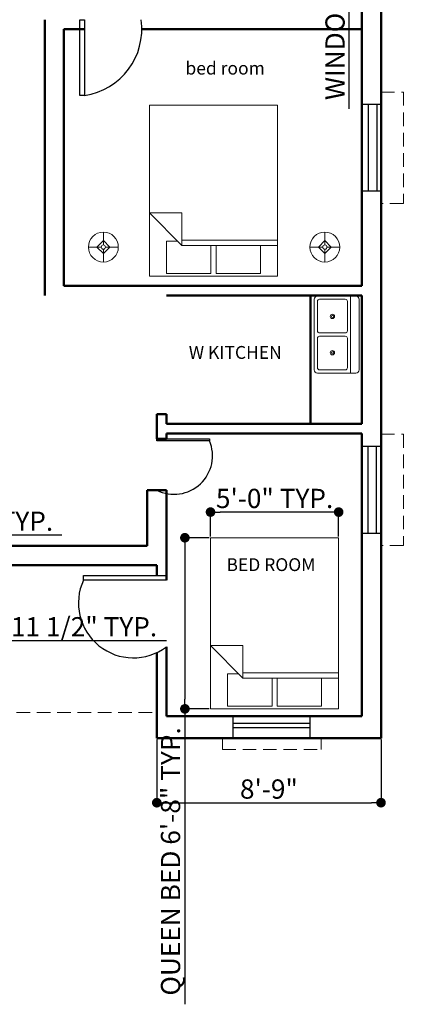
# Model space of a CAD drawing. Units: inches. Extents: x 2050 to 6806, y 2092 to 5743.
# Tile 5 of 8: x 3382 to 3567, y 2211 to 2671. Entities that reach past the tile are written whole.
import ezdxf

# ---------------------------------------------------------------- set-up
doc = ezdxf.new("R2010")
doc.units = ezdxf.units.IN
doc.linetypes.add('HIDDEN', pattern=[9.525, 6.35, -3.175])
for name, color, linetype, lineweight in [('A-ANNO-DIMS', 2, 'Continuous', 18), ('A-AREA-IDEN', 7, 'Continuous', 18), ('A-DOOR', 2, 'Continuous', 25), ('A-FLOR-FIXT', 4, 'Continuous', 18), ('A-FLOR-OVHD', 30, 'HIDDEN', 18), ('A-FURN', 5, 'Continuous', 18), ('A-GLAZ', 6, 'Continuous', 25), ('A-WALL', 7, 'Continuous', 50)]:
    doc.layers.add(name, color=color, linetype=linetype, lineweight=lineweight)
doc.styles.get("Standard").update_dxf_attribs({"font": 'arial.ttf'})
doc.dimstyles.new('ISO-25', dxfattribs={"dimtxt": 9, "dimasz": 4.5, "dimexe": 1.25, "dimexo": 0.625, "dimtad": 1, "dimdec": 1, "dimlunit": 4, "dimtxsty": 'Standard', "dimblk": 'DOT', "dimcen": 2.5, "dimadec": 0, "dimazin": 0, "dimtfac": 1, "dimtdec": 1, "dimtmove": 0, "dimatfit": 3, "dimldrblk": 'ARCHTICK', "dimfxl": 1, "dimarcsym": 0})

# ---------------------------------------------------------------- blocks, each defined once
blk = doc.blocks.new('Bed - Queen')
for p, q in [((0, -80.00003), (0, 0)), ((0, 0), (59.99999, 0)), ((59.99999, 0), (59.99999, -80.00003)), ((7.99999, -1.2), (28.79998, -1.2)), ((7.99999, -14.4), (7.99999, -1.2)), ((28.79998, -1.2), (28.79998, -14.4)), ((31.19999, -1.2), (51.99999, -1.2)), ((31.19999, -14.4), (31.19999, -1.2)), ((51.99999, -1.2), (51.99999, -16.4)), ((0, -14.4), (44.8, -14.4)), ((44.8, -16.8), (0, -16.8)), ((59.99999, -29.6), (44.8, -14.4)), ((44.8, -14.4), (44.8, -29.6)), ((51.99999, -16.4), (46.79936, -16.4)), ((44.8, -29.6), (59.99999, -29.6)), ((59.99999, -80.00003), (0, -80.00003))]:
    blk.add_line(p, q)
blk = doc.blocks.new('Lamp - Table')
for p, q in [((0, 7), (0, 1)), ((-1, 0), (-7, 0)), ((0, 3), (-3, 0)), ((-3, 0), (0, -3)), ((3, 0), (0, 3)), ((0, -3), (3, 0)), ((1, 0), (7, 0)), ((0, -1), (0, -7))]:
    blk.add_line(p, q)
for radius in [7, 1]:
    blk.add_circle((0, 0), radius)
blk = doc.blocks.new('Sink-double - 36 in top')
for p, q in [((-18, -4), (18, -4)), ((-0.75, -18.5), (-0.75, -6.5)), ((0.75, -6.5), (0.75, -18.5))]:
    blk.add_line(p, q)
for points in [[(-16.5, 0), (16.5, 0)], [(-18, -19.5), (-18, -1.5)], [(18, -1.5), (18, -19.5)], [(-16.5, -18.5), (-16.5, -6.5)], [(-15.5, -5.5), (-1.75, -5.5)], [(1.75, -5.5), (15.5, -5.5)], [(16.5, -6.5), (16.5, -18.5)], [(16.5, -21), (-16.5, -21)], [(-1.75, -19.5), (-15.5, -19.5)], [(15.5, -19.5), (1.75, -19.5)]]:
    blk.add_lwpolyline(points)
for centre, radius in [((-8.5, -12.5), 1), ((-8.5, -12.5), 0.5), ((8.5, -12.5), 1), ((8.5, -12.5), 0.5)]:
    blk.add_circle(centre, radius)
for centre, radius, start, end in [((-16.5, -1.5), 1.5, 90, 180), ((16.5, -1.5), 1.5, 0, 90), ((-15.5, -6.5), 1, 90, 180), ((-1.75, -6.5), 1, 0, 90), ((1.75, -6.5), 1, 90, 180), ((15.5, -6.5), 1, 0, 90), ((-16.5, -19.5), 1.5, 180, 270), ((-15.5, -18.5), 1, 180, 270), ((-1.75, -18.5), 1, 270, 0), ((1.75, -18.5), 1, 180, 270), ((15.5, -18.5), 1, 270, 0), ((16.5, -19.5), 1.5, 270, 0)]:
    blk.add_arc(centre, radius, start, end)
blk = doc.blocks.new('_Dot')
at = {"color": 0, "linetype": 'ByBlock', "lineweight": -2}
blk.add_line((-0.5, 0), (-1, 0), dxfattribs=at)
at = {"color": 0, "linetype": 'ByBlock', "const_width": 0.5}
blk.add_lwpolyline([(-0.25, 0, 1), (0.25, 0, 1)], format="xyb", close=True, dxfattribs=at)
blk = doc.blocks.new('*D43')
at = {"layer": 'A-ANNO-DIMS', "color": 0, "lineweight": -2, "transparency": 16777216}
for p, q in [((3446.67, 2334.81), (3446.67, 2303.96)), ((3551.67, 2334.81), (3551.67, 2303.96)), ((3451.17, 2305.21), (3547.17, 2305.21))]:
    blk.add_line(p, q, dxfattribs=at)
at = {"layer": 'Defpoints', "color": 0, "transparency": 16777216}
for p in [(3446.67, 2335.44), (3551.67, 2335.44), (3551.67, 2305.21)]:
    blk.add_point(p, dxfattribs=at)
at = {"layer": 'A-ANNO-DIMS', "color": 0, "lineweight": -2, "transparency": 16777216, "xscale": 4.5, "yscale": 4.5, "zscale": 4.5, "rotation": 180}
blk.add_blockref('_Dot', (3446.67, 2305.21), dxfattribs=at)
at = {"layer": 'A-ANNO-DIMS', "color": 0, "lineweight": -2, "transparency": 16777216, "xscale": 4.5, "yscale": 4.5, "zscale": 4.5}
blk.add_blockref('_Dot', (3551.67, 2305.21), dxfattribs=at)
at = {"layer": 'A-ANNO-DIMS', "color": 0, "transparency": 16777216, "insert": (3499.17, 2310.43), "char_height": 9, "attachment_point": 5}
blk.add_mtext('8\'-9"', dxfattribs=at)
blk = doc.blocks.new('_ArchTick')
at = {"color": 0, "linetype": 'ByBlock', "const_width": 0.15}
blk.add_lwpolyline([(-0.5, -0.5), (0.5, 0.5)], dxfattribs=at)
blk = doc.blocks.new('DOOR-750')
blk.add_lwpolyline([(28.97, 0), (26.83, 0), (26.83, 35.38), (28.97, 35.38)], close=True)
blk.add_arc((31.25, 4.42), 31.27, 98.1233, 188.1233)
blk = doc.blocks.new('WIN-1050')
for p, q in [((0, 40.58), (9, 40.58)), ((2.5, 0), (2.5, 40.58)), ((6.5, 0), (6.5, 40.58)), ((0, 0), (9, 0))]:
    blk.add_line(p, q)
blk = doc.blocks.new('SUNSHADE-A')
for p, q in [((0, 52.08), (10.45, 52.08)), ((10.45, 52.08), (10.45, 0)), ((10.45, 0), (0, 0))]:
    blk.add_line(p, q)
blk = doc.blocks.new('*D65')
at = {"layer": 'A-ANNO-DIMS', "color": 0, "lineweight": -2, "transparency": 16777216}
for p, q in [((3471.21, 2429.09), (3458.58, 2429.09)), ((3459.83, 2424.59), (3459.83, 2353.59)), ((3471.21, 2349.09), (3458.58, 2349.09)), ((3459.83, 2349.09), (3459.83, 2210.95))]:
    blk.add_line(p, q, dxfattribs=at)
at = {"layer": 'Defpoints', "color": 0, "transparency": 16777216}
for p in [(3471.83, 2429.09), (3459.83, 2349.09), (3471.83, 2349.09)]:
    blk.add_point(p, dxfattribs=at)
at = {"layer": 'A-ANNO-DIMS', "color": 0, "lineweight": -2, "transparency": 16777216, "xscale": 4.5, "yscale": 4.5, "zscale": 4.5}
for p, rotation in [((3459.83, 2429.09), 90), ((3459.83, 2349.09), 270)]:
    blk.add_blockref('_Dot', p, dxfattribs=dict(at, rotation=rotation))
at = {"layer": 'A-ANNO-DIMS', "color": 0, "transparency": 16777216, "insert": (3454.28, 2277.77), "char_height": 9, "attachment_point": 5, "rotation": 90}
blk.add_mtext('QUEEN BED 6\'-8" TYP.', dxfattribs=at)
blk = doc.blocks.new('*D66')
at = {"layer": 'A-ANNO-DIMS', "color": 0, "lineweight": -2, "transparency": 16777216}
for p, q in [((3471.83, 2429.71), (3471.83, 2442.34)), ((3527.33, 2441.09), (3476.33, 2441.09)), ((3531.83, 2429.71), (3531.83, 2442.34))]:
    blk.add_line(p, q, dxfattribs=at)
at = {"layer": 'Defpoints', "color": 0, "transparency": 16777216}
for p in [(3471.83, 2441.09), (3471.83, 2429.09), (3531.83, 2429.09)]:
    blk.add_point(p, dxfattribs=at)
at = {"layer": 'A-ANNO-DIMS', "color": 0, "lineweight": -2, "transparency": 16777216, "xscale": 4.5, "yscale": 4.5, "zscale": 4.5, "rotation": 180}
blk.add_blockref('_Dot', (3471.83, 2441.09), dxfattribs=at)
at = {"layer": 'A-ANNO-DIMS', "color": 0, "lineweight": -2, "transparency": 16777216, "xscale": 4.5, "yscale": 4.5, "zscale": 4.5}
blk.add_blockref('_Dot', (3531.83, 2441.09), dxfattribs=at)
at = {"layer": 'A-ANNO-DIMS', "color": 0, "transparency": 16777216, "insert": (3501.83, 2446.31), "char_height": 9, "attachment_point": 5}
blk.add_mtext('5\'-0" TYP.', dxfattribs=at)
blk = doc.blocks.new('*D67')
at = {"layer": 'A-ANNO-DIMS', "color": 0, "lineweight": -2, "transparency": 16777216}
for p, q in [((3542.05, 2854.17), (3535.33, 2854.17)), ((3536.58, 2849.67), (3536.58, 2818.09)), ((3542.05, 2813.59), (3535.33, 2813.59)), ((3536.58, 2813.59), (3536.58, 2629.65))]:
    blk.add_line(p, q, dxfattribs=at)
at = {"layer": 'Defpoints', "color": 0, "transparency": 16777216}
for p in [(3542.67, 2854.17), (3536.58, 2813.59), (3542.67, 2813.59)]:
    blk.add_point(p, dxfattribs=at)
at = {"layer": 'A-ANNO-DIMS', "color": 0, "lineweight": -2, "transparency": 16777216, "xscale": 4.5, "yscale": 4.5, "zscale": 4.5}
for p, rotation in [((3536.58, 2854.17), 90), ((3536.58, 2813.59), 270)]:
    blk.add_blockref('_Dot', p, dxfattribs=dict(at, rotation=rotation))
at = {"layer": 'A-ANNO-DIMS', "color": 0, "transparency": 16777216, "insert": (3531.3, 2719.37), "char_height": 9, "attachment_point": 5, "rotation": 90}
blk.add_mtext('WINDOW W1050 3\'-4 1/2" TYP.', dxfattribs=at)
blk = doc.blocks.new('*D77')
at = {"layer": 'A-ANNO-DIMS', "color": 0, "lineweight": -2, "transparency": 16777216}
for p, q in [((3231.3, 2385.71), (3231.3, 2379.77)), ((3266.67, 2385.71), (3266.67, 2379.77)), ((3235.8, 2381.02), (3262.17, 2381.02)), ((3266.67, 2381.02), (3451.21, 2381.02))]:
    blk.add_line(p, q, dxfattribs=at)
at = {"layer": 'Defpoints', "color": 0, "transparency": 16777216}
for p in [(3231.3, 2386.33), (3266.67, 2386.33), (3266.67, 2381.02)]:
    blk.add_point(p, dxfattribs=at)
at = {"layer": 'A-ANNO-DIMS', "color": 0, "lineweight": -2, "transparency": 16777216, "xscale": 4.5, "yscale": 4.5, "zscale": 4.5, "rotation": 180}
blk.add_blockref('_Dot', (3231.3, 2381.02), dxfattribs=at)
at = {"layer": 'A-ANNO-DIMS', "color": 0, "lineweight": -2, "transparency": 16777216, "xscale": 4.5, "yscale": 4.5, "zscale": 4.5}
blk.add_blockref('_Dot', (3266.67, 2381.02), dxfattribs=at)
at = {"layer": 'A-ANNO-DIMS', "color": 0, "transparency": 16777216, "insert": (3361.19, 2386.31), "char_height": 9, "attachment_point": 5}
blk.add_mtext('DOUBLE DOOR 2\'-11 1/2" TYP.', dxfattribs=at)
blk = doc.blocks.new('*D99')
at = {"layer": 'A-ANNO-DIMS', "color": 0, "lineweight": -2, "transparency": 16777216}
for p, q in [((3236.22, 2433.21), (3236.22, 2429.14)), ((3259.22, 2433.21), (3259.22, 2429.14)), ((3240.72, 2430.39), (3254.72, 2430.39)), ((3259.22, 2430.39), (3402.15, 2430.39))]:
    blk.add_line(p, q, dxfattribs=at)
at = {"layer": 'Defpoints', "color": 0, "transparency": 16777216}
for p in [(3236.22, 2433.84), (3259.22, 2433.84), (3259.22, 2430.39)]:
    blk.add_point(p, dxfattribs=at)
at = {"layer": 'A-ANNO-DIMS', "color": 0, "lineweight": -2, "transparency": 16777216, "xscale": 4.5, "yscale": 4.5, "zscale": 4.5, "rotation": 180}
blk.add_blockref('_Dot', (3236.22, 2430.39), dxfattribs=at)
at = {"layer": 'A-ANNO-DIMS', "color": 0, "lineweight": -2, "transparency": 16777216, "xscale": 4.5, "yscale": 4.5, "zscale": 4.5}
blk.add_blockref('_Dot', (3259.22, 2430.39), dxfattribs=at)
at = {"layer": 'A-ANNO-DIMS', "color": 0, "transparency": 16777216, "insert": (3332.93, 2435.67), "char_height": 9, "attachment_point": 5}
blk.add_mtext('COMPUTER 1\'-11" TYP.', dxfattribs=at)

msp = doc.modelspace()

# ---------------------------------------------------------------- linework, layer by layer
at = {"layer": 'A-DOOR'}
for points in [[(3446.67, 2475.33), (3471.32, 2475.33), (3471.32, 2474.49), (3446.67, 2474.49)], [(3451.17, 2409.33), (3412.31, 2409.33), (3412.31, 2411.46), (3451.17, 2411.46)]]:
    msp.add_lwpolyline(points, close=True, dxfattribs=at)
for centre, radius, start, end in [((3454.75, 2467.43), 18.02, 243.3595, 23.0612), ((3435.69, 2398.64), 25.7, 155.4184, 307.0519)]:
    msp.add_arc(centre, radius, start, end, dxfattribs=at)
at = {"layer": 'A-FLOR-OVHD'}
for p, q in [((3551.67, 2335.44), (3551.67, 2416.33)), ((3266.67, 2347.33), (3446.67, 2347.33)), ((3446.67, 2335.44), (3551.67, 2335.44)), ((3477.37, 2335.44), (3477.37, 2330.06)), ((3523.62, 2330.06), (3523.62, 2335.44)), ((3477.37, 2330.06), (3523.62, 2330.06))]:
    msp.add_line(p, q, dxfattribs=at)
at = {"layer": 'A-GLAZ'}
for p, q in [((3482.28, 2345.7), (3482.28, 2335.44)), ((3518.28, 2345.7), (3518.28, 2335.44)), ((3518.28, 2342.2), (3482.28, 2342.2)), ((3518.28, 2340.2), (3482.28, 2340.2)), ((3518.28, 2340.2), (3482.28, 2340.2))]:
    msp.add_line(p, q, dxfattribs=at)
at = {"layer": 'A-WALL'}
for p, q in [((3551.67, 2416.33), (3551.67, 2881.33)), ((3542.67, 2546.83), (3542.67, 2719.33)), ((3394.17, 2671.33), (3394.17, 2542.33)), ((3403.17, 2666.83), (3403.17, 2546.83)), ((3412.81, 2666.83), (3403.17, 2666.83)), ((3466.17, 2666.83), (3439.66, 2666.83)), ((3542.67, 2666.83), (3466.17, 2666.83)), ((3542.67, 2546.83), (3403.17, 2546.83)), ((3542.67, 2546.83), (3466.17, 2546.83)), ((3542.67, 2542.33), (3451.17, 2542.33)), ((3518.67, 2482.33), (3518.67, 2542.33)), ((3542.67, 2482.33), (3542.67, 2542.33)), ((3446.67, 2486.83), (3451.17, 2486.83)), ((3446.67, 2475.33), (3446.67, 2486.83)), ((3451.17, 2482.33), (3451.17, 2486.83)), ((3542.67, 2482.33), (3451.17, 2482.33)), ((3542.67, 2477.83), (3451.17, 2477.83)), ((3451.17, 2475.33), (3451.17, 2477.83)), ((3451.17, 2475.33), (3451.17, 2477.83)), ((3542.67, 2345.7), (3542.67, 2477.83)), ((3446.67, 2475.33), (3451.17, 2475.33)), ((3442.17, 2451.33), (3451.17, 2451.33)), ((3442.17, 2425.33), (3442.17, 2451.33)), ((3451.17, 2420.83), (3451.17, 2451.33)), ((3451.17, 2420.83), (3451.17, 2451.33)), ((3271.17, 2425.33), (3442.17, 2425.33)), ((3451.17, 2420.83), (3451.17, 2409.33)), ((3266.67, 2416.33), (3446.67, 2416.33)), ((3446.67, 2416.33), (3446.67, 2411.46)), ((3542.67, 2416.33), (3542.67, 2345.7)), ((3551.67, 2416.33), (3551.67, 2335.44)), ((3451.17, 2378.13), (3451.17, 2345.7)), ((3446.67, 2375.41), (3446.67, 2335.44)), ((3542.67, 2345.7), (3451.17, 2345.7)), ((3551.67, 2335.44), (3446.67, 2335.44))]:
    msp.add_line(p, q, dxfattribs=at)
msp.add_lwpolyline([(3551.67, 2345.7), (3551.67, 2335.44), (3542.67, 2335.44)], dxfattribs=at)

# ---------------------------------------------------------------- block references
at = {"layer": 'A-DOOR', "rotation": 180}
msp.add_blockref('DOOR-750', (3439.64, 2671.33), dxfattribs=at)
at = {"layer": 'A-FLOR-FIXT', "rotation": 270}
msp.add_blockref('Sink-double - 36 in top', (3541.41, 2524.1), dxfattribs=at)
at = {"layer": 'A-FLOR-OVHD'}
for p in [(3551.67, 2585.4), (3551.67, 2425.43)]:
    msp.add_blockref('SUNSHADE-A', p, dxfattribs=at)
at = {"layer": 'A-FURN', "rotation": 180}
for p in [(3503.24, 2551.38), (3531.83, 2349.09)]:
    msp.add_blockref('Bed - Queen', p, dxfattribs=at)
at = {"layer": 'A-FURN'}
for p in [(3421.65, 2565.02), (3525.36, 2565.02)]:
    msp.add_blockref('Lamp - Table', p, dxfattribs=at)
at = {"layer": 'A-GLAZ', "rotation": 180}
for p in [(3552.14, 2631.69), (3551.97, 2471.74)]:
    msp.add_blockref('WIN-1050', p, dxfattribs=at)

# ---------------------------------------------------------------- texts
at = {"layer": 'A-AREA-IDEN'}
for s, p in [('bed room', (3460.08, 2645.67)), ('W KITCHEN', (3461.65, 2512.75)), ('BED ROOM', (3479.3, 2413.52))]:
    msp.add_text(s, height=6, dxfattribs=at).set_placement(p)

# ---------------------------------------------------------------- dimensions: what is measured, and where the dimension line sits
at = {"layer": 'A-ANNO-DIMS'}
for base, p1, p2, angle, text, picture, middle in [((3536.58, 2813.59), (3542.67, 2854.17), (3542.67, 2813.59), 270, 'WINDOW W1050 <> TYP.', '*D67', (3531.3, 2719.37)), ((3471.83, 2441.09), (3531.83, 2429.09), (3471.83, 2429.09), 180, '<> TYP.', '*D66', (3501.83, 2446.31)), ((3459.83, 2349.09), (3471.83, 2429.09), (3471.83, 2349.09), 270, 'QUEEN BED <> TYP.', '*D65', (3454.28, 2277.77))]:
    dim = msp.add_linear_dim(base=base, p1=p1, p2=p2, angle=angle, text=text, dimstyle='ISO-25', override={"dimdec": 1, "dimlfac": 1, "dimrnd": 0, "dimzin": 1, "dimdsep": 46, "dimlunit": 4, "dimfrac": 2}, dxfattribs=at)
    dim.commit()
    dim.dimension.update_dxf_attribs({"geometry": picture, "text_midpoint": middle})
for base, p1, p2, text, picture, middle in [((3259.22, 2430.39), (3236.22, 2433.84), (3259.22, 2433.84), 'COMPUTER <> TYP.', '*D99', (3332.93, 2435.67)), ((3266.67, 2381.02), (3231.3, 2386.33), (3266.67, 2386.33), 'DOUBLE DOOR <> TYP.', '*D77', (3361.19, 2386.31))]:
    dim = msp.add_linear_dim(base=base, p1=p1, p2=p2, text=text, dimstyle='ISO-25', override={"dimdec": 1, "dimlfac": 1, "dimrnd": 0, "dimzin": 1, "dimdsep": 46, "dimlunit": 4, "dimfrac": 2}, dxfattribs=at)
    dim.commit()
    dim.dimension.update_dxf_attribs({"geometry": picture, "text_midpoint": middle})
dim = msp.add_linear_dim(base=(3551.67, 2305.21), p1=(3446.67, 2335.44), p2=(3551.67, 2335.44), dimstyle='ISO-25', override={"dimclrd": 0, "dimclre": 0, "dimclrt": 0}, dxfattribs=at)
dim.commit()
dim.dimension.update_dxf_attribs({"geometry": '*D43', "text_midpoint": (3499.17, 2310.43)})

doc.saveas('drawing.dxf')
